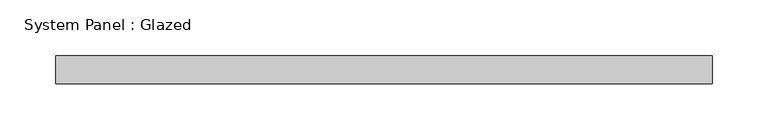
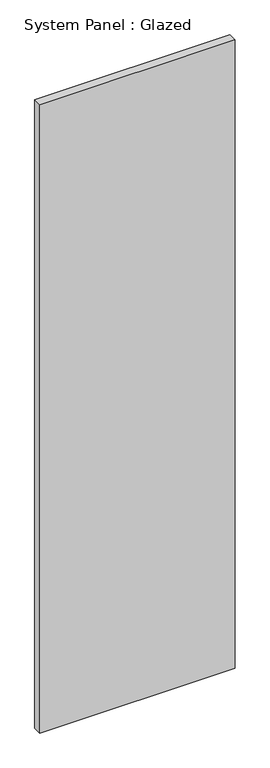
"""IFC4 building model written with IfcOpenShell, lengths in millimetres: plate geometry, System Panel : Glazed."""

from ifc_helpers import new_model, si_unit, origin, origin_with_axes, place, context, project, spatial, polyline, outline, extrude, source, transform, mapped, element, save


def system_panel_glazed_29c37de9(model_context):
    return source(origin(), model_context, "Body", "SweptSolid", [
        extrude(outline(polyline([(295.275, 19.05), (-295.275, 19.05), (-295.275, 44.45), (295.275, 44.45), (295.275, 19.05)])), origin_with_axes(), (0.0, 0.0, 1.0), 2006.6),
    ])


if __name__ == "__main__":
    model = new_model("IFC4")
    model_context = context("Model", 3, world=origin())
    ifc_project = project(units=[si_unit("LENGTHUNIT", "METRE", prefix="MILLI")], contexts=[model_context])
    site = spatial("IfcSite", under=ifc_project)
    building = spatial("IfcBuilding", under=site)
    placement = place(None, origin())
    system_panel_glazed_shape = system_panel_glazed_29c37de9(model_context)
    element("IfcPlate", 1, ObjectType="System Panel : Glazed", at=placement, inside=building, context=model_context, shape_type="MappedRepresentation", body=[
        mapped(system_panel_glazed_shape, transform((0.0, 0.0, 0.0), x_axis=(1.0, 0.0, 0.0), y_axis=(0.0, 1.0, 0.0), z_axis=(0.0, 0.0, 1.0))),
    ])
    save(model, "model.ifc")

# Revit data of these elements
# Type "System Panel : Glazed"
#   Construction Type Id = "GSP4R"
#   Analytic Construction = "1/8 in Pilkington single glazing"
#   Visual Light Transmittance = 0.9
#   Solar Heat Gain Coefficient = 0.86
#   Heat Transfer Coefficient (U) = 1.18115 BTU/(h·ft²·°F)
#   Define Thermal Properties by = 1
# Element 1 (IfcPlate, "System Panel : Glazed")
#   Materials on its faces: "Glass"
# Materials
#   "Glass": class "Glass", colour RGB 0 128 192, transparency 0.75, Description = "Soda Lime Glass", Cost = 0
